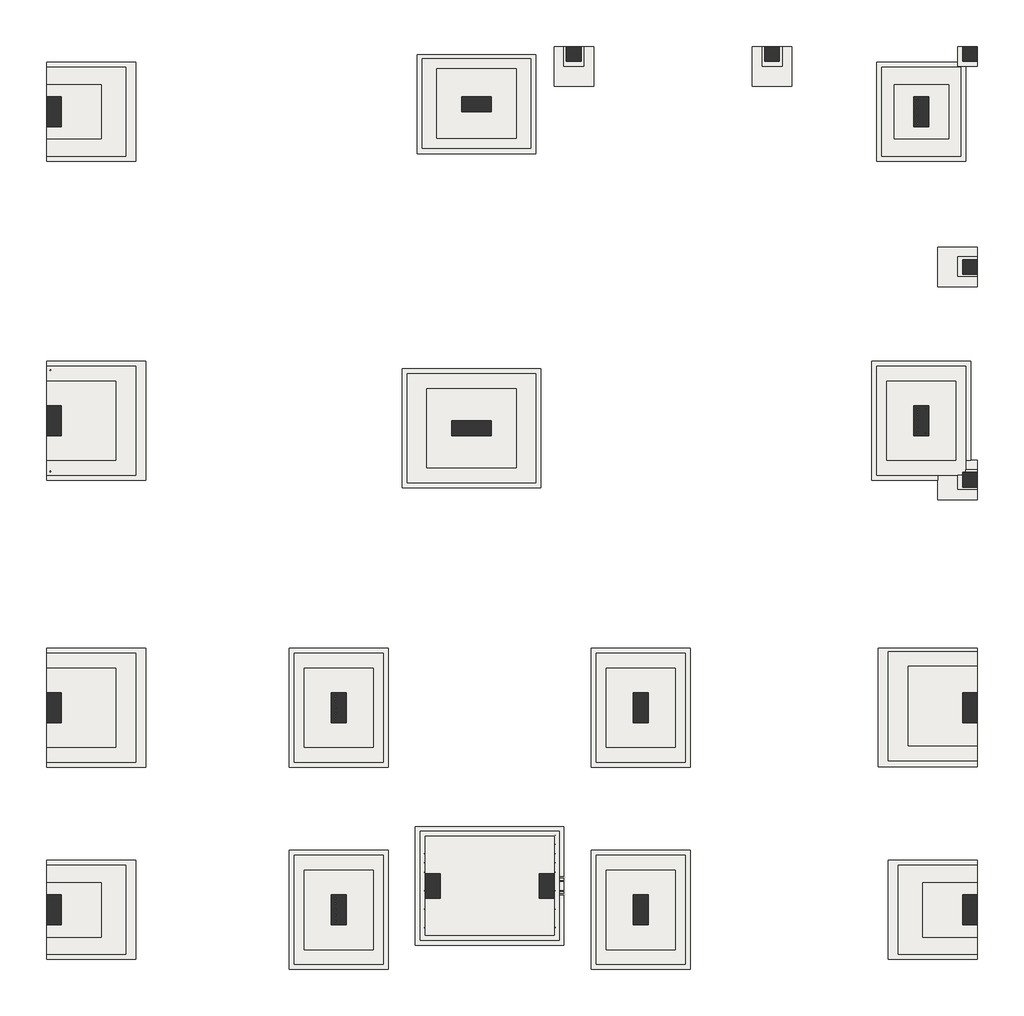
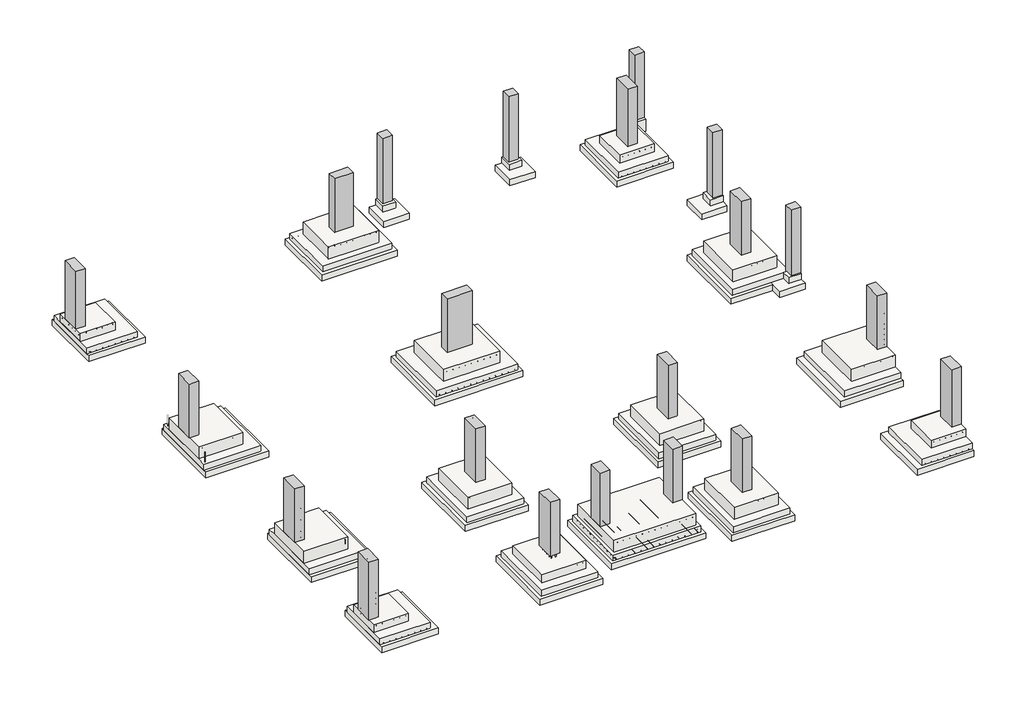
# One storey, part 1 of 6: 38 slabs, 21 columns.
"""IFC4 building model written with IfcOpenShell, lengths in millimetres."""

from ifc_helpers import new_model, si_unit, frame, origin, place, context, project, spatial, polyline, outline, extrude, faceted_brep, transform, mapped, element, save
from components import concrete_rectangular_column_c_1fc459bc

model = new_model("IFC4")

# Units and contexts
model_context = context("Model", 3, world=origin())
ifc_project = project(units=[si_unit("LENGTHUNIT", "METRE", prefix="MILLI")], contexts=[model_context])

# Site, building, storey
site = spatial("IfcSite", under=ifc_project)
building = spatial("IfcBuilding", under=site)
storey = spatial("IfcBuildingStorey", under=building, Elevation=-1828.8)

# Columns
placement = place(None, origin())
concrete_rectangular_column_c_shape = concrete_rectangular_column_c_1fc459bc(model_context)
element("IfcColumn", 1, ObjectType="Concrete-Rectangular-Column : C", at=placement, inside=storey, context=model_context, shape_type="MappedRepresentation", body=[
    mapped(concrete_rectangular_column_c_shape, transform((5670699.8650571, -3584604.6060698, 0.0), x_axis=(1.0, 0.0, 0.0), y_axis=(0.0, 1.0, 0.0), z_axis=(0.0, 0.0, 1.0))),
])
element("IfcColumn", 2, ObjectType="Concrete-Rectangular-Column : C", at=placement, inside=storey, context=model_context, shape_type="MappedRepresentation", body=[
    mapped(concrete_rectangular_column_c_shape, transform((5673747.8650571, -3584604.6060698, 0.0), x_axis=(1.0, 0.0, 0.0), y_axis=(0.0, 1.0, 0.0), z_axis=(0.0, 0.0, 1.0))),
])
element("IfcColumn", 3, ObjectType="Concrete-Rectangular-Column : C", at=placement, inside=storey, context=model_context, shape_type="MappedRepresentation", body=[
    mapped(concrete_rectangular_column_c_shape, transform((5676795.8650571, -3584604.6060698, 0.0), x_axis=(1.0, 0.0, 0.0), y_axis=(0.0, 1.0, 0.0), z_axis=(0.0, 0.0, 1.0))),
])
element("IfcColumn", 4, ObjectType="Concrete-Rectangular-Column : C", at=placement, inside=storey, context=model_context, shape_type="MappedRepresentation", body=[
    mapped(concrete_rectangular_column_c_shape, transform((5676795.8650571, -3587881.949152, 0.0), x_axis=(1.0, 0.0, 0.0), y_axis=(0.0, 1.0, 0.0), z_axis=(0.0, 0.0, 1.0))),
])
element("IfcColumn", 5, ObjectType="Concrete-Rectangular-Column : C", at=placement, inside=storey, context=model_context, shape_type="MappedRepresentation", body=[
    mapped(concrete_rectangular_column_c_shape, transform((5676795.8650571, -3591159.3007286, 0.0), x_axis=(1.0, 0.0, 0.0), y_axis=(0.0, 1.0, 0.0), z_axis=(0.0, 0.0, 1.0))),
])
element("IfcColumn", 6, ObjectType="Concrete-Rectangular-Column : C1", at=placement, inside=storey, context=model_context, shape_type="SweptSolid", body=[
    extrude(outline(polyline([(5662813.1113073, -3585265.1289932), (5662813.1113073, -3585722.3289932), (5662584.5113073, -3585722.3289932), (5662584.5113073, -3585265.1289932), (5662813.1113073, -3585265.1289932)])), frame((0.0, 0.0, -1473.2), z_axis=(0.0, 0.0, 1.0), x_axis=(1.0, 0.0, 0.0)), (0.0, 0.0, 1.0), 1473.2),
])
element("IfcColumn", 7, ObjectType="Concrete-Rectangular-Column : C1", at=placement, inside=storey, context=model_context, shape_type="SweptSolid", body=[
    extrude(outline(polyline([(5676160.8165246, -3585265.1224803), (5676160.8165246, -3585722.3224803), (5675932.2165246, -3585722.3224803), (5675932.2165246, -3585265.1224803), (5676160.8165246, -3585265.1224803)])), frame((0.0, 0.0, -1473.2), z_axis=(0.0, 0.0, 1.0), x_axis=(1.0, 0.0, 0.0)), (0.0, 0.0, 1.0), 1473.2),
])
element("IfcColumn", 8, ObjectType="Concrete-Rectangular-Column : C1", at=placement, inside=storey, context=model_context, shape_type="SweptSolid", body=[
    extrude(outline(polyline([(5662813.1113073, -3597545.8975754), (5662813.1113073, -3598003.0975754), (5662584.5113073, -3598003.0975754), (5662584.5113073, -3597545.8975754), (5662813.1113073, -3597545.8975754)])), frame((0.0, 0.0, -1473.2), z_axis=(0.0, 0.0, 1.0), x_axis=(1.0, 0.0, 0.0)), (0.0, 0.0, 1.0), 1473.2),
])
element("IfcColumn", 9, ObjectType="Concrete-Rectangular-Column : C1", at=placement, inside=storey, context=model_context, shape_type="SweptSolid", body=[
    extrude(outline(polyline([(5676910.1113073, -3597545.8975754), (5676910.1113073, -3598003.0975754), (5676681.5113073, -3598003.0975754), (5676681.5113073, -3597545.8975754), (5676910.1113073, -3597545.8975754)])), frame((0.0, 0.0, -1473.2), z_axis=(0.0, 0.0, 1.0), x_axis=(1.0, 0.0, 0.0)), (0.0, 0.0, 1.0), 1473.2),
])
element("IfcColumn", 10, ObjectType="Concrete-Rectangular-Column : C2", at=placement, inside=storey, context=model_context, shape_type="SweptSolid", body=[
    extrude(outline(polyline([(5668972.6206949, -3585265.1224803), (5669429.8206949, -3585265.1224803), (5669429.8206949, -3585493.7224803), (5668972.6206949, -3585493.7224803), (5668972.6206949, -3585265.1224803)])), frame((0.0, 0.0, -1371.6), z_axis=(0.0, 0.0, 1.0), x_axis=(1.0, 0.0, 0.0)), (0.0, 0.0, 1.0), 1371.6),
])
element("IfcColumn", 11, ObjectType="Concrete-Rectangular-Column : C2", at=placement, inside=storey, context=model_context, shape_type="SweptSolid", body=[
    extrude(outline(polyline([(5676160.8165246, -3590021.0682909), (5676160.8165246, -3590478.2682909), (5675932.2165246, -3590478.2682909), (5675932.2165246, -3590021.0682909), (5676160.8165246, -3590021.0682909)])), frame((0.0, 0.0, -1371.6), z_axis=(0.0, 0.0, 1.0), x_axis=(1.0, 0.0, 0.0)), (0.0, 0.0, 1.0), 1371.6),
])
element("IfcColumn", 12, ObjectType="Concrete-Rectangular-Column : C2", at=placement, inside=storey, context=model_context, shape_type="SweptSolid", body=[
    extrude(outline(polyline([(5662813.1650571, -3590021.0682909), (5662813.1650571, -3590478.2682909), (5662584.5650571, -3590478.2682909), (5662584.5650571, -3590021.0682909), (5662813.1650571, -3590021.0682909)])), frame((0.0, 0.0, -1371.6), z_axis=(0.0, 0.0, 1.0), x_axis=(1.0, 0.0, 0.0)), (0.0, 0.0, 1.0), 1371.6),
])
element("IfcColumn", 13, ObjectType="Concrete-Rectangular-Column : C2", at=placement, inside=storey, context=model_context, shape_type="SweptSolid", body=[
    extrude(outline(polyline([(5662813.1650571, -3594436.6523052), (5662813.1650571, -3594893.8523052), (5662584.5650571, -3594893.8523052), (5662584.5650571, -3594436.6523052), (5662813.1650571, -3594436.6523052)])), frame((0.0, 0.0, -1371.6), z_axis=(0.0, 0.0, 1.0), x_axis=(1.0, 0.0, 0.0)), (0.0, 0.0, 1.0), 1371.6),
])
element("IfcColumn", 14, ObjectType="Concrete-Rectangular-Column : C2", at=placement, inside=storey, context=model_context, shape_type="SweptSolid", body=[
    extrude(outline(polyline([(5667194.6165246, -3594436.6523052), (5667194.6165246, -3594893.8523052), (5666966.0165246, -3594893.8523052), (5666966.0165246, -3594436.6523052), (5667194.6165246, -3594436.6523052)])), frame((0.0, 0.0, -1371.6), z_axis=(0.0, 0.0, 1.0), x_axis=(1.0, 0.0, 0.0)), (0.0, 0.0, 1.0), 1371.6),
])
element("IfcColumn", 15, ObjectType="Concrete-Rectangular-Column : C2", at=placement, inside=storey, context=model_context, shape_type="SweptSolid", body=[
    extrude(outline(polyline([(5671842.8165246, -3594436.6523052), (5671842.8165246, -3594893.8523052), (5671614.2165246, -3594893.8523052), (5671614.2165246, -3594436.6523052), (5671842.8165246, -3594436.6523052)])), frame((0.0, 0.0, -1371.6), z_axis=(0.0, 0.0, 1.0), x_axis=(1.0, 0.0, 0.0)), (0.0, 0.0, 1.0), 1371.6),
])
element("IfcColumn", 16, ObjectType="Concrete-Rectangular-Column : C2", at=placement, inside=storey, context=model_context, shape_type="SweptSolid", body=[
    extrude(outline(polyline([(5676910.1650571, -3594436.6523052), (5676910.1650571, -3594893.8523052), (5676681.5650571, -3594893.8523052), (5676681.5650571, -3594436.6523052), (5676910.1650571, -3594436.6523052)])), frame((0.0, 0.0, -1371.6), z_axis=(0.0, 0.0, 1.0), x_axis=(1.0, 0.0, 0.0)), (0.0, 0.0, 1.0), 1371.6),
])
element("IfcColumn", 17, ObjectType="Concrete-Rectangular-Column : C2", at=placement, inside=storey, context=model_context, shape_type="SweptSolid", body=[
    extrude(outline(polyline([(5671842.8165246, -3597545.8975754), (5671842.8165246, -3598003.0975754), (5671614.2165246, -3598003.0975754), (5671614.2165246, -3597545.8975754), (5671842.8165246, -3597545.8975754)])), frame((0.0, 0.0, -1371.6), z_axis=(0.0, 0.0, 1.0), x_axis=(1.0, 0.0, 0.0)), (0.0, 0.0, 1.0), 1371.6),
])
element("IfcColumn", 18, ObjectType="Concrete-Rectangular-Column : C2", at=placement, inside=storey, context=model_context, shape_type="SweptSolid", body=[
    extrude(outline(polyline([(5667194.6165246, -3597545.8975754), (5667194.6165246, -3598003.0975754), (5666966.0165246, -3598003.0975754), (5666966.0165246, -3597545.8975754), (5667194.6165246, -3597545.8975754)])), frame((0.0, 0.0, -1371.6), z_axis=(0.0, 0.0, 1.0), x_axis=(1.0, 0.0, 0.0)), (0.0, 0.0, 1.0), 1371.6),
])
element("IfcColumn", 19, ObjectType="Concrete-Rectangular-Column : C3", at=placement, inside=storey, context=model_context, shape_type="SweptSolid", body=[
    extrude(outline(polyline([(5668820.2206949, -3590249.6682909), (5669429.8206949, -3590249.6682909), (5669429.8206949, -3590478.2682909), (5668820.2206949, -3590478.2682909), (5668820.2206949, -3590249.6682909)])), frame((0.0, 0.0, -1371.6), z_axis=(0.0, 0.0, 1.0), x_axis=(1.0, 0.0, 0.0)), (0.0, 0.0, 1.0), 1371.6),
])
element("IfcColumn", 20, ObjectType="Concrete-Rectangular-Column : C4", at=placement, inside=storey, context=model_context, shape_type="SweptSolid", body=[
    extrude(outline(polyline([(5668642.4165246, -3597217.2875145), (5668642.4165246, -3597598.2875145), (5668413.8165246, -3597598.2875145), (5668413.8165246, -3597217.2875145), (5668642.4165246, -3597217.2875145)])), frame((0.0, 0.0, -1371.6), z_axis=(0.0, 0.0, 1.0), x_axis=(1.0, 0.0, 0.0)), (0.0, 0.0, 1.0), 1371.6),
])
element("IfcColumn", 21, ObjectType="Concrete-Rectangular-Column : C4", at=placement, inside=storey, context=model_context, shape_type="SweptSolid", body=[
    extrude(outline(polyline([(5670395.0165245, -3597217.2875145), (5670395.0165245, -3597598.2875145), (5670166.4165245, -3597598.2875145), (5670166.4165245, -3597217.2875145), (5670395.0165245, -3597217.2875145)])), frame((0.0, 0.0, -1371.6), z_axis=(0.0, 0.0, 1.0), x_axis=(1.0, 0.0, 0.0)), (0.0, 0.0, 1.0), 1371.6),
])

# Slabs
element("IfcSlab", 22, ObjectType="Footing-Rectangular : F1", at=placement, inside=storey, context=model_context, shape_type="Brep", body=[
    faceted_brep([(5663803.7113073, -3584807.9113604, -1676.4), (5662584.5113073, -3584807.9113604, -1676.4), (5662584.5113073, -3585074.6113604, -1676.4), (5662584.5113073, -3585912.8113604, -1676.4), (5662584.5113073, -3586179.5113604, -1676.4), (5663803.7113073, -3586179.5113604, -1676.4), (5663803.7113073, -3584807.9113604, -1828.8), (5662584.5113073, -3584807.9113604, -1828.8), (5662584.5113073, -3586179.5113604, -1828.8), (5663803.7113073, -3586179.5113604, -1828.8)], [[[0, 1, 2, 3, 4, 5]], [[1, 0, 6, 7]], [[4, 3, 2, 1, 7, 8]], [[5, 4, 8, 9]], [[0, 5, 9, 6]], [[7, 6, 9, 8]]]),
])
element("IfcSlab", 23, ObjectType="Footing-Rectangular : F1", at=placement, inside=storey, context=model_context, shape_type="SweptSolid", body=[
    extrude(outline(polyline([(5675436.9165246, -3584807.9224803), (5676656.1165246, -3584807.9224803), (5676656.1165246, -3586179.5224803), (5675436.9165246, -3586179.5224803), (5675436.9165246, -3584807.9224803)])), frame((0.0, 0.0, -1828.8), z_axis=(0.0, 0.0, 1.0), x_axis=(1.0, 0.0, 0.0)), (0.0, 0.0, 1.0), 152.4),
])
element("IfcSlab", 24, ObjectType="Footing-Rectangular : F1", at=placement, inside=storey, context=model_context, shape_type="Brep", body=[
    faceted_brep([(5663803.7113073, -3597090.2875145, -1676.4), (5662584.5113073, -3597090.2875145, -1676.4), (5662584.5113073, -3597356.9875145, -1676.4), (5662584.5113073, -3598195.1875145, -1676.4), (5662584.5113073, -3598461.8875145, -1676.4), (5663803.7113073, -3598461.8875145, -1676.4), (5663803.7113073, -3597090.2875145, -1828.8), (5662584.5113073, -3597090.2875145, -1828.8), (5662584.5113073, -3598461.8875145, -1828.8), (5663803.7113073, -3598461.8875145, -1828.8)], [[[0, 1, 2, 3, 4, 5]], [[1, 0, 6, 7]], [[4, 3, 2, 1, 7, 8]], [[5, 4, 8, 9]], [[0, 5, 9, 6]], [[7, 6, 9, 8]]]),
])
element("IfcSlab", 25, ObjectType="Footing-Rectangular : F1", at=placement, inside=storey, context=model_context, shape_type="Brep", body=[
    faceted_brep([(5676910.1650571, -3597090.2875145, -1676.4), (5675690.9650571, -3597090.2875145, -1676.4), (5675690.9650571, -3598461.8875145, -1676.4), (5676910.1650571, -3598461.8875145, -1676.4), (5676910.1650571, -3598195.1875145, -1676.4), (5676910.1650571, -3597356.9875145, -1676.4), (5676910.1650571, -3597090.2875145, -1828.8), (5675690.9650571, -3597090.2875145, -1828.8), (5675690.9650571, -3598461.8875145, -1828.8), (5676910.1650571, -3598461.8875145, -1828.8)], [[[0, 1, 2, 3, 4, 5]], [[1, 0, 6, 7]], [[2, 1, 7, 8]], [[3, 2, 8, 9]], [[0, 5, 4, 3, 9, 6]], [[7, 6, 9, 8]]]),
])
element("IfcSlab", 26, ObjectType="Footing-Rectangular : F1 TOP", at=placement, inside=storey, context=model_context, shape_type="SweptSolid", body=[
    extrude(outline(polyline([(5662584.5113073, -3585074.6113604), (5663422.7113073, -3585074.6113604), (5663422.7113073, -3585912.8113604), (5662584.5113073, -3585912.8113604), (5662584.5113073, -3585074.6113604)])), frame((0.0, 0.0, -1676.4), z_axis=(0.0, 0.0, 1.0), x_axis=(1.0, 0.0, 0.0)), (0.0, 0.0, 1.0), 203.2),
])
element("IfcSlab", 27, ObjectType="Footing-Rectangular : F1 TOP", at=placement, inside=storey, context=model_context, shape_type="SweptSolid", body=[
    extrude(outline(polyline([(5675627.4165246, -3585912.8224803), (5675627.4165246, -3585074.6224803), (5676465.6165246, -3585074.6224803), (5676465.6165246, -3585912.8224803), (5675627.4165246, -3585912.8224803)])), frame((0.0, 0.0, -1676.4), z_axis=(0.0, 0.0, 1.0), x_axis=(1.0, 0.0, 0.0)), (0.0, 0.0, 1.0), 203.2),
])
element("IfcSlab", 28, ObjectType="Footing-Rectangular : F1 TOP", at=placement, inside=storey, context=model_context, shape_type="SweptSolid", body=[
    extrude(outline(polyline([(5662584.5113073, -3597356.9875145), (5663422.7113073, -3597356.9875145), (5663422.7113073, -3598195.1875145), (5662584.5113073, -3598195.1875145), (5662584.5113073, -3597356.9875145)])), frame((0.0, 0.0, -1676.4), z_axis=(0.0, 0.0, 1.0), x_axis=(1.0, 0.0, 0.0)), (0.0, 0.0, 1.0), 203.2),
])
element("IfcSlab", 29, ObjectType="Footing-Rectangular : F1 TOP", at=placement, inside=storey, context=model_context, shape_type="SweptSolid", body=[
    extrude(outline(polyline([(5676071.9650571, -3598195.1875145), (5676071.9650571, -3597356.9875145), (5676910.1650571, -3597356.9875145), (5676910.1650571, -3598195.1875145), (5676071.9650571, -3598195.1875145)])), frame((0.0, 0.0, -1676.4), z_axis=(0.0, 0.0, 1.0), x_axis=(1.0, 0.0, 0.0)), (0.0, 0.0, 1.0), 203.2),
])
element("IfcSlab", 30, ObjectType="Footing-Rectangular : F2", at=placement, inside=storey, context=model_context, shape_type="SweptSolid", body=[
    extrude(outline(polyline([(5668363.0297535, -3586052.5224803), (5668363.0297535, -3584680.9224803), (5670039.4297535, -3584680.9224803), (5670039.4297535, -3586052.5224803), (5668363.0297535, -3586052.5224803)])), frame((0.0, 0.0, -1828.8), z_axis=(0.0, 0.0, 1.0), x_axis=(1.0, 0.0, 0.0)), (0.0, 0.0, 1.0), 152.4),
])
element("IfcSlab", 31, ObjectType="Footing-Rectangular : F2", at=placement, inside=storey, context=model_context, shape_type="Brep", body=[
    faceted_brep([(5663956.1113073, -3589411.5284482, -1676.4), (5662584.5113073, -3589411.5284482, -1676.4), (5662584.5113073, -3589640.1284482, -1676.4), (5662584.5113073, -3590859.3284482, -1676.4), (5662584.5113073, -3591087.9284482, -1676.4), (5663956.1113073, -3591087.9284482, -1676.4), (5663956.1113073, -3589411.5284482, -1828.8), (5662584.5113073, -3589411.5284482, -1828.8), (5662584.5113073, -3591087.9284482, -1828.8), (5663956.1113073, -3591087.9284482, -1828.8)], [[[0, 1, 2, 3, 4, 5]], [[1, 0, 6, 7]], [[4, 3, 2, 1, 7, 8]], [[5, 4, 8, 9]], [[0, 5, 9, 6]], [[7, 6, 9, 8]]]),
])
element("IfcSlab", 32, ObjectType="Footing-Rectangular : F2", at=placement, inside=storey, context=model_context, shape_type="Brep", body=[
    faceted_brep([(5676732.3165246, -3589411.4682909, -1676.4), (5675360.7165246, -3589411.4682909, -1676.4), (5675360.7165246, -3591087.8682909, -1676.4), (5676605.3650571, -3591087.8682909, -1676.4), (5676732.3165246, -3591087.8682909, -1676.4), (5676732.3165246, -3591000.363802, -1676.4), (5676732.3165246, -3589411.4682909, -1828.8), (5675360.7165246, -3589411.4682909, -1828.8), (5675360.7165246, -3591087.8682909, -1828.8), (5676605.3650571, -3591087.8682909, -1828.8), (5676732.3165246, -3591087.8682909, -1828.8), (5676732.3165246, -3591000.363802, -1828.8)], [[[0, 1, 2, 3, 4, 5]], [[1, 0, 6, 7]], [[2, 1, 7, 8]], [[4, 3, 2, 8, 9, 10]], [[0, 5, 4, 10, 11, 6]], [[7, 6, 11, 10, 9, 8]]]),
])
element("IfcSlab", 33, ObjectType="Footing-Rectangular : F2", at=placement, inside=storey, context=model_context, shape_type="Brep", body=[
    faceted_brep([(5663956.1113073, -3593827.0523052, -1676.4), (5662584.5113073, -3593827.0523052, -1676.4), (5662584.5113073, -3594055.6523052, -1676.4), (5662584.5113073, -3595274.8523052, -1676.4), (5662584.5113073, -3595503.4523052, -1676.4), (5663956.1113073, -3595503.4523052, -1676.4), (5663956.1113073, -3593827.0523052, -1828.8), (5662584.5113073, -3593827.0523052, -1828.8), (5662584.5113073, -3595503.4523052, -1828.8), (5663956.1113073, -3595503.4523052, -1828.8)], [[[0, 1, 2, 3, 4, 5]], [[1, 0, 6, 7]], [[4, 3, 2, 1, 7, 8]], [[5, 4, 8, 9]], [[0, 5, 9, 6]], [[7, 6, 9, 8]]]),
])
element("IfcSlab", 34, ObjectType="Footing-Rectangular : F2", at=placement, inside=storey, context=model_context, shape_type="SweptSolid", body=[
    extrude(outline(polyline([(5666394.5165246, -3596937.8875145), (5667766.1165246, -3596937.8875145), (5667766.1165246, -3598614.2875145), (5666394.5165246, -3598614.2875145), (5666394.5165246, -3596937.8875145)])), frame((0.0, 0.0, -1828.8), z_axis=(0.0, 0.0, 1.0), x_axis=(1.0, 0.0, 0.0)), (0.0, 0.0, 1.0), 152.4),
])
element("IfcSlab", 35, ObjectType="Footing-Rectangular : F2", at=placement, inside=storey, context=model_context, shape_type="SweptSolid", body=[
    extrude(outline(polyline([(5671042.7165246, -3596937.8875145), (5672414.3165246, -3596937.8875145), (5672414.3165246, -3598614.2875145), (5671042.7165246, -3598614.2875145), (5671042.7165246, -3596937.8875145)])), frame((0.0, 0.0, -1828.8), z_axis=(0.0, 0.0, 1.0), x_axis=(1.0, 0.0, 0.0)), (0.0, 0.0, 1.0), 152.4),
])
element("IfcSlab", 36, ObjectType="Footing-Rectangular : F2", at=placement, inside=storey, context=model_context, shape_type="Brep", body=[
    faceted_brep([(5676910.1650571, -3593801.6523052, -1676.4), (5675538.5650571, -3593801.6523052, -1676.4), (5675538.5650571, -3595478.0523052, -1676.4), (5676910.1650571, -3595478.0523052, -1676.4), (5676910.1650571, -3595249.4523052, -1676.4), (5676910.1650571, -3594030.2523052, -1676.4), (5676910.1650571, -3593801.6523052, -1828.8), (5675538.5650571, -3593801.6523052, -1828.8), (5675538.5650571, -3595478.0523052, -1828.8), (5676910.1650571, -3595478.0523052, -1828.8)], [[[0, 1, 2, 3, 4, 5]], [[1, 0, 6, 7]], [[2, 1, 7, 8]], [[3, 2, 8, 9]], [[0, 5, 4, 3, 9, 6]], [[7, 6, 9, 8]]]),
])
element("IfcSlab", 37, ObjectType="Footing-Rectangular : F2", at=placement, inside=storey, context=model_context, shape_type="SweptSolid", body=[
    extrude(outline(polyline([(5666394.5165246, -3593827.0523052), (5667766.1165246, -3593827.0523052), (5667766.1165246, -3595503.4523052), (5666394.5165246, -3595503.4523052), (5666394.5165246, -3593827.0523052)])), frame((0.0, 0.0, -1828.8), z_axis=(0.0, 0.0, 1.0), x_axis=(1.0, 0.0, 0.0)), (0.0, 0.0, 1.0), 152.4),
])
element("IfcSlab", 38, ObjectType="Footing-Rectangular : F2", at=placement, inside=storey, context=model_context, shape_type="SweptSolid", body=[
    extrude(outline(polyline([(5671042.7165246, -3593827.0523052), (5672414.3165246, -3593827.0523052), (5672414.3165246, -3595503.4523052), (5671042.7165246, -3595503.4523052), (5671042.7165246, -3593827.0523052)])), frame((0.0, 0.0, -1828.8), z_axis=(0.0, 0.0, 1.0), x_axis=(1.0, 0.0, 0.0)), (0.0, 0.0, 1.0), 152.4),
])
element("IfcSlab", 39, ObjectType="Footing-Rectangular : F2 TOP", at=placement, inside=storey, context=model_context, shape_type="SweptSolid", body=[
    extrude(outline(polyline([(5668591.6297535, -3585900.1224803), (5668591.6297535, -3584833.3224803), (5669810.8297535, -3584833.3224803), (5669810.8297535, -3585900.1224803), (5668591.6297535, -3585900.1224803)])), frame((0.0, 0.0, -1676.4), z_axis=(0.0, 0.0, 1.0), x_axis=(1.0, 0.0, 0.0)), (0.0, 0.0, 1.0), 304.8),
])
element("IfcSlab", 40, ObjectType="Footing-Rectangular : F2 TOP", at=placement, inside=storey, context=model_context, shape_type="SweptSolid", body=[
    extrude(outline(polyline([(5663651.3113073, -3590859.3284482), (5662584.5113073, -3590859.3284482), (5662584.5113073, -3589640.1284482), (5663651.3113073, -3589640.1284482), (5663651.3113073, -3590859.3284482)])), frame((0.0, 0.0, -1676.4), z_axis=(0.0, 0.0, 1.0), x_axis=(1.0, 0.0, 0.0)), (0.0, 0.0, 1.0), 304.8),
])
element("IfcSlab", 41, ObjectType="Footing-Rectangular : F2 TOP", at=placement, inside=storey, context=model_context, shape_type="SweptSolid", body=[
    extrude(outline(polyline([(5675513.1165246, -3589640.0682909), (5676579.9165246, -3589640.0682909), (5676579.9165246, -3590859.2682909), (5675513.1165246, -3590859.2682909), (5675513.1165246, -3589640.0682909)])), frame((0.0, 0.0, -1676.4), z_axis=(0.0, 0.0, 1.0), x_axis=(1.0, 0.0, 0.0)), (0.0, 0.0, 1.0), 304.8),
])
element("IfcSlab", 42, ObjectType="Footing-Rectangular : F2 TOP", at=placement, inside=storey, context=model_context, shape_type="SweptSolid", body=[
    extrude(outline(polyline([(5662584.5113073, -3594055.6523052), (5663651.3113073, -3594055.6523052), (5663651.3113073, -3595274.8523052), (5662584.5113073, -3595274.8523052), (5662584.5113073, -3594055.6523052)])), frame((0.0, 0.0, -1676.4), z_axis=(0.0, 0.0, 1.0), x_axis=(1.0, 0.0, 0.0)), (0.0, 0.0, 1.0), 304.8),
])
element("IfcSlab", 43, ObjectType="Footing-Rectangular : F2 TOP", at=placement, inside=storey, context=model_context, shape_type="SweptSolid", body=[
    extrude(outline(polyline([(5666546.9165246, -3597166.4875145), (5667613.7165246, -3597166.4875145), (5667613.7165246, -3598385.6875145), (5666546.9165246, -3598385.6875145), (5666546.9165246, -3597166.4875145)])), frame((0.0, 0.0, -1676.4), z_axis=(0.0, 0.0, 1.0), x_axis=(1.0, 0.0, 0.0)), (0.0, 0.0, 1.0), 203.2),
])
element("IfcSlab", 44, ObjectType="Footing-Rectangular : F2 TOP", at=placement, inside=storey, context=model_context, shape_type="SweptSolid", body=[
    extrude(outline(polyline([(5671195.1165246, -3597166.4875145), (5672261.9165246, -3597166.4875145), (5672261.9165246, -3598385.6875145), (5671195.1165246, -3598385.6875145), (5671195.1165246, -3597166.4875145)])), frame((0.0, 0.0, -1676.4), z_axis=(0.0, 0.0, 1.0), x_axis=(1.0, 0.0, 0.0)), (0.0, 0.0, 1.0), 304.8),
])
element("IfcSlab", 45, ObjectType="Footing-Rectangular : F2 TOP", at=placement, inside=storey, context=model_context, shape_type="SweptSolid", body=[
    extrude(outline(polyline([(5675843.3650571, -3594030.2523052), (5676910.1650571, -3594030.2523052), (5676910.1650571, -3595249.4523052), (5675843.3650571, -3595249.4523052), (5675843.3650571, -3594030.2523052)])), frame((0.0, 0.0, -1676.4), z_axis=(0.0, 0.0, 1.0), x_axis=(1.0, 0.0, 0.0)), (0.0, 0.0, 1.0), 304.8),
])
element("IfcSlab", 46, ObjectType="Footing-Rectangular : F2 TOP", at=placement, inside=storey, context=model_context, shape_type="SweptSolid", body=[
    extrude(outline(polyline([(5666546.9165246, -3594055.6523052), (5667613.7165246, -3594055.6523052), (5667613.7165246, -3595274.8523052), (5666546.9165246, -3595274.8523052), (5666546.9165246, -3594055.6523052)])), frame((0.0, 0.0, -1676.4), z_axis=(0.0, 0.0, 1.0), x_axis=(1.0, 0.0, 0.0)), (0.0, 0.0, 1.0), 304.8),
])
element("IfcSlab", 47, ObjectType="Footing-Rectangular : F2 TOP", at=placement, inside=storey, context=model_context, shape_type="SweptSolid", body=[
    extrude(outline(polyline([(5671195.1165246, -3594055.6523052), (5672261.9165246, -3594055.6523052), (5672261.9165246, -3595274.8523052), (5671195.1165246, -3595274.8523052), (5671195.1165246, -3594055.6523052)])), frame((0.0, 0.0, -1676.4), z_axis=(0.0, 0.0, 1.0), x_axis=(1.0, 0.0, 0.0)), (0.0, 0.0, 1.0), 304.8),
])
element("IfcSlab", 48, ObjectType="Footing-Rectangular : F3", at=placement, inside=storey, context=model_context, shape_type="SweptSolid", body=[
    extrude(outline(polyline([(5668134.4297535, -3591202.2284482), (5668134.4297535, -3589525.8284482), (5670115.6297535, -3589525.8284482), (5670115.6297535, -3591202.2284482), (5668134.4297535, -3591202.2284482)])), frame((0.0, 0.0, -1828.8), z_axis=(0.0, 0.0, 1.0), x_axis=(1.0, 0.0, 0.0)), (0.0, 0.0, 1.0), 152.4),
])
element("IfcSlab", 49, ObjectType="Footing-Rectangular : F3 TOP", at=placement, inside=storey, context=model_context, shape_type="SweptSolid", body=[
    extrude(outline(polyline([(5668439.2297535, -3590973.6284482), (5668439.2297535, -3589754.4284482), (5669810.8297535, -3589754.4284482), (5669810.8297535, -3590973.6284482), (5668439.2297535, -3590973.6284482)])), frame((0.0, 0.0, -1676.4), z_axis=(0.0, 0.0, 1.0), x_axis=(1.0, 0.0, 0.0)), (0.0, 0.0, 1.0), 304.8),
])
element("IfcSlab", 50, ObjectType="Footing-Rectangular : F4", at=placement, inside=storey, context=model_context, shape_type="SweptSolid", body=[
    extrude(outline(polyline([(5668337.6165246, -3598245.9875145), (5668337.6165246, -3596569.5875145), (5670471.2165246, -3596569.5875145), (5670471.2165246, -3598245.9875145), (5668337.6165246, -3598245.9875145)])), frame((0.0, 0.0, -1828.8), z_axis=(0.0, 0.0, 1.0), x_axis=(1.0, 0.0, 0.0)), (0.0, 0.0, 1.0), 152.4),
])
element("IfcSlab", 51, ObjectType="Footing-Rectangular : F4 TOP", at=placement, inside=storey, context=model_context, shape_type="SweptSolid", body=[
    extrude(outline(polyline([(5668413.8165246, -3598169.7875145), (5668413.8165246, -3596645.7875145), (5670395.0165246, -3596645.7875145), (5670395.0165246, -3598169.7875145), (5668413.8165246, -3598169.7875145)])), frame((0.0, 0.0, -1676.4), z_axis=(0.0, 0.0, 1.0), x_axis=(1.0, 0.0, 0.0)), (0.0, 0.0, 1.0), 304.8),
])
element("IfcSlab", 52, ObjectType="Footing-Rectangular : FOOTING", at=placement, inside=storey, context=model_context, shape_type="SweptSolid", body=[
    extrude(outline(polyline([(5670547.4297535, -3584490.4224803), (5670852.2297535, -3584490.4224803), (5670852.2297535, -3584795.2224803), (5670547.4297535, -3584795.2224803), (5670547.4297535, -3584490.4224803)])), frame((0.0, 0.0, -1828.8), z_axis=(0.0, 0.0, 1.0), x_axis=(1.0, 0.0, 0.0)), (0.0, 0.0, 1.0), 152.4),
])
element("IfcSlab", 53, ObjectType="Footing-Rectangular : FOOTING", at=placement, inside=storey, context=model_context, shape_type="SweptSolid", body=[
    extrude(outline(polyline([(5673602.0019836, -3584490.4224803), (5673906.8019836, -3584490.4224803), (5673906.8019836, -3584795.2224803), (5673602.0019836, -3584795.2224803), (5673602.0019836, -3584490.4224803)])), frame((0.0, 0.0, -1828.8), z_axis=(0.0, 0.0, 1.0), x_axis=(1.0, 0.0, 0.0)), (0.0, 0.0, 1.0), 152.4),
])
element("IfcSlab", 54, ObjectType="Footing-Rectangular : FOOTING", at=placement, inside=storey, context=model_context, shape_type="SweptSolid", body=[
    extrude(outline(polyline([(5676605.3650571, -3587723.0122254), (5676910.1650571, -3587723.0122254), (5676910.1650571, -3588027.8122254), (5676605.3650571, -3588027.8122254), (5676605.3650571, -3587723.0122254)])), frame((0.0, 0.0, -1828.8), z_axis=(0.0, 0.0, 1.0), x_axis=(1.0, 0.0, 0.0)), (0.0, 0.0, 1.0), 152.4),
])
element("IfcSlab", 55, ObjectType="Footing-Rectangular : FOOTING", at=placement, inside=storey, context=model_context, shape_type="SweptSolid", body=[
    extrude(outline(polyline([(5676732.3165246, -3591000.363802), (5676910.1650571, -3591000.363802), (5676910.1650571, -3591305.163802), (5676605.3650571, -3591305.163802), (5676605.3650571, -3591087.8682909), (5676732.3165246, -3591087.8682909), (5676732.3165246, -3591000.363802)])), frame((0.0, 0.0, -1828.8), z_axis=(0.0, 0.0, 1.0), x_axis=(1.0, 0.0, 0.0)), (0.0, 0.0, 1.0), 152.4),
])
element("IfcSlab", 56, ObjectType="Footing-Rectangular : FOOTING", at=placement, inside=storey, context=model_context, shape_type="Brep", body=[
    faceted_brep([(5676910.1650571, -3584490.4224803, -1676.4), (5676605.3650571, -3584490.4224803, -1676.4), (5676605.3650571, -3584795.2224803, -1676.4), (5676910.1650571, -3584795.2224803, -1676.4), (5676910.1650571, -3584490.4224803, -1981.2), (5676910.1650571, -3584795.2224803, -1981.2), (5676732.3165246, -3584795.2224803, -1981.2), (5676732.3165246, -3584731.7289932, -1981.2), (5676605.3650571, -3584731.7289932, -1981.2), (5676605.3650571, -3584490.4224803, -1981.2), (5676605.3650571, -3584731.7289932, -1828.8), (5676605.3650571, -3584795.2224803, -1828.8), (5676732.3165246, -3584795.2224803, -1828.8), (5676732.3165246, -3584731.7289932, -1828.8)], [[[0, 1, 2, 3]], [[4, 5, 6, 7, 8, 9]], [[1, 0, 4, 9]], [[2, 1, 9, 8, 10, 11]], [[3, 2, 11, 12, 6, 5]], [[0, 3, 5, 4]], [[13, 12, 11, 10]], [[13, 7, 6, 12]], [[7, 13, 10, 8]]]),
])
element("IfcSlab", 57, ObjectType="PCC", at=placement, inside=storey, context=model_context, shape_type="Brep", body=[
    faceted_brep([(5663956.1113073, -3584731.7113604, -1981.2), (5663956.1113073, -3586255.7113604, -1981.2), (5662584.5113073, -3586255.7113604, -1981.2), (5662584.5113073, -3584731.7113604, -1981.2), (5663956.1113073, -3584731.7113604, -1828.8), (5662584.5113073, -3584731.7113604, -1828.8), (5662584.5113073, -3584807.9113604, -1828.8), (5662584.5113073, -3586179.5113604, -1828.8), (5662584.5113073, -3586255.7113604, -1828.8), (5663956.1113073, -3586255.7113604, -1828.8)], [[[0, 1, 2, 3]], [[4, 5, 6, 7, 8, 9]], [[1, 0, 4, 9]], [[2, 1, 9, 8]], [[3, 2, 8, 7, 6, 5]], [[0, 3, 5, 4]]]),
])
element("IfcSlab", 58, ObjectType="PCC", at=placement, inside=storey, context=model_context, shape_type="Brep", body=[
    faceted_brep([(5670115.6206949, -3584617.4224803, -1981.2), (5670115.6206949, -3586141.4224803, -1981.2), (5668286.8206949, -3586141.4224803, -1981.2), (5668286.8206949, -3584617.4224803, -1981.2), (5670115.6206949, -3584617.4224803, -1828.8), (5668286.8206949, -3584617.4224803, -1828.8), (5668286.8206949, -3586141.4224803, -1828.8), (5670115.6206949, -3586141.4224803, -1828.8)], [[[0, 1, 2, 3]], [[4, 5, 6, 7]], [[1, 0, 4, 7]], [[2, 1, 7, 6]], [[3, 2, 6, 5]], [[0, 3, 5, 4]]]),
    faceted_brep([(5675284.5165246, -3591164.0682909, -1981.2), (5675284.5165246, -3589335.2682909, -1981.2), (5676808.5165246, -3589335.2682909, -1981.2), (5676808.5165246, -3590854.4964814, -1981.2), (5676300.8086455, -3590854.4964814, -1981.2), (5676300.8086455, -3591164.0682909, -1981.2), (5676300.5650571, -3591164.0682909, -1981.2), (5675284.5165246, -3591164.0682909, -1828.8), (5676300.5650571, -3591164.0682909, -1828.8), (5676300.8086455, -3591164.0682909, -1828.8), (5676300.8086455, -3590854.4964814, -1828.8), (5676808.5165246, -3590854.4964814, -1828.8), (5676808.5165246, -3589335.2682909, -1828.8), (5675284.5165246, -3589335.2682909, -1828.8)], [[[0, 1, 2, 3, 4, 5, 6]], [[7, 8, 9, 10, 11, 12, 13]], [[1, 0, 7, 13]], [[2, 1, 13, 12]], [[3, 2, 12, 11]], [[0, 6, 5, 9, 8, 7]], [[4, 3, 11, 10]], [[5, 4, 10, 9]]]),
    faceted_brep([(5675386.1650571, -3595575.3283721, -1981.2), (5675386.1650571, -3593746.5283721, -1981.2), (5676910.1650571, -3593746.5283721, -1981.2), (5676910.1650571, -3595575.3283721, -1981.2), (5675386.1650571, -3595575.3283721, -1828.8), (5676910.1650571, -3595575.3283721, -1828.8), (5676910.1650571, -3595478.0523052, -1828.8), (5676910.1650571, -3593801.6523052, -1828.8), (5676910.1650571, -3593746.5283721, -1828.8), (5675386.1650571, -3593746.5283721, -1828.8)], [[[0, 1, 2, 3]], [[4, 5, 6, 7, 8, 9]], [[1, 0, 4, 9]], [[2, 1, 9, 8]], [[3, 2, 8, 7, 6, 5]], [[0, 3, 5, 4]]]),
    faceted_brep([(5676910.1650571, -3597008.3822736, -1981.2), (5676910.1650571, -3598532.3822736, -1981.2), (5675538.0601964, -3598532.3822736, -1981.2), (5675538.0601964, -3597008.3822736, -1981.2), (5676910.1650571, -3597008.3822736, -1828.8), (5675538.0601964, -3597008.3822736, -1828.8), (5675538.0601964, -3598532.3822736, -1828.8), (5676910.1650571, -3598532.3822736, -1828.8), (5676910.1650571, -3598461.8875145, -1828.8), (5676910.1650571, -3597090.2875145, -1828.8)], [[[0, 1, 2, 3]], [[4, 5, 6, 7, 8, 9]], [[1, 0, 4, 9, 8, 7]], [[2, 1, 7, 6]], [[3, 2, 6, 5]], [[0, 3, 5, 4]]]),
    faceted_brep([(5672490.5165246, -3596860.0975754, -1981.2), (5672490.5165246, -3598688.8975754, -1981.2), (5670966.5165246, -3598688.8975754, -1981.2), (5670966.5165246, -3596860.0975754, -1981.2), (5672490.5165246, -3596860.0975754, -1828.8), (5670966.5165246, -3596860.0975754, -1828.8), (5670966.5165246, -3598688.8975754, -1828.8), (5672490.5165246, -3598688.8975754, -1828.8)], [[[0, 1, 2, 3]], [[4, 5, 6, 7]], [[1, 0, 4, 7]], [[2, 1, 7, 6]], [[3, 2, 6, 5]], [[0, 3, 5, 4]]]),
    faceted_brep([(5672490.5165246, -3593750.8523052, -1981.2), (5672490.5165246, -3595579.6523052, -1981.2), (5670966.5165246, -3595579.6523052, -1981.2), (5670966.5165246, -3593750.8523052, -1981.2), (5672490.5165246, -3593750.8523052, -1828.8), (5670966.5165246, -3593750.8523052, -1828.8), (5670966.5165246, -3595579.6523052, -1828.8), (5672490.5165246, -3595579.6523052, -1828.8)], [[[0, 1, 2, 3]], [[4, 5, 6, 7]], [[1, 0, 4, 7]], [[2, 1, 7, 6]], [[3, 2, 6, 5]], [[0, 3, 5, 4]]]),
    faceted_brep([(5668261.4165246, -3598322.1875145, -1981.2), (5668261.4165246, -3596493.3875145, -1981.2), (5670547.4165246, -3596493.3875145, -1981.2), (5670547.4165246, -3598322.1875145, -1981.2), (5668261.4165246, -3598322.1875145, -1828.8), (5670547.4165246, -3598322.1875145, -1828.8), (5670547.4165246, -3596493.3875145, -1828.8), (5668261.4165246, -3596493.3875145, -1828.8)], [[[0, 1, 2, 3]], [[4, 5, 6, 7]], [[1, 0, 4, 7]], [[2, 1, 7, 6]], [[3, 2, 6, 5]], [[0, 3, 5, 4]]]),
    faceted_brep([(5667842.3165246, -3596860.0975754, -1981.2), (5667842.3165246, -3598688.8975754, -1981.2), (5666318.3165246, -3598688.8975754, -1981.2), (5666318.3165246, -3596860.0975754, -1981.2), (5667842.3165246, -3596860.0975754, -1828.8), (5666318.3165246, -3596860.0975754, -1828.8), (5666318.3165246, -3598688.8975754, -1828.8), (5667842.3165246, -3598688.8975754, -1828.8)], [[[0, 1, 2, 3]], [[4, 5, 6, 7]], [[1, 0, 4, 7]], [[2, 1, 7, 6]], [[3, 2, 6, 5]], [[0, 3, 5, 4]]]),
    faceted_brep([(5662584.5113073, -3598536.5187088, -1981.2), (5662584.5113073, -3597012.5187088, -1981.2), (5663956.1650571, -3597012.5187088, -1981.2), (5663956.1650571, -3598536.5187088, -1981.2), (5662584.5113073, -3598536.5187088, -1828.8), (5663956.1650571, -3598536.5187088, -1828.8), (5663956.1650571, -3597012.5187088, -1828.8), (5662584.5113073, -3597012.5187088, -1828.8), (5662584.5113073, -3597090.2875145, -1828.8), (5662584.5113073, -3598461.8875145, -1828.8)], [[[0, 1, 2, 3]], [[4, 5, 6, 7, 8, 9]], [[1, 0, 4, 9, 8, 7]], [[2, 1, 7, 6]], [[3, 2, 6, 5]], [[0, 3, 5, 4]]]),
    faceted_brep([(5662584.5113073, -3595579.7655499, -1981.2), (5662584.5113073, -3593750.9655499, -1981.2), (5664108.5650571, -3593750.9655499, -1981.2), (5664108.5650571, -3595579.7655499, -1981.2), (5662584.5113073, -3595579.7655499, -1828.8), (5664108.5650571, -3595579.7655499, -1828.8), (5664108.5650571, -3593750.9655499, -1828.8), (5662584.5113073, -3593750.9655499, -1828.8), (5662584.5113073, -3593827.0523052, -1828.8), (5662584.5113073, -3595503.4523052, -1828.8)], [[[0, 1, 2, 3]], [[4, 5, 6, 7, 8, 9]], [[1, 0, 4, 9, 8, 7]], [[2, 1, 7, 6]], [[3, 2, 6, 5]], [[0, 3, 5, 4]]]),
    faceted_brep([(5662584.5113073, -3591164.0682909, -1981.2), (5662584.5113073, -3589335.2682909, -1981.2), (5664108.5650571, -3589335.2682909, -1981.2), (5664108.5650571, -3591164.0682909, -1981.2), (5662584.5113073, -3591164.0682909, -1828.8), (5664108.5650571, -3591164.0682909, -1828.8), (5664108.5650571, -3589335.2682909, -1828.8), (5662584.5113073, -3589335.2682909, -1828.8), (5662584.5113073, -3589411.5284482, -1828.8), (5662584.5113073, -3591087.9284482, -1828.8)], [[[0, 1, 2, 3]], [[4, 5, 6, 7, 8, 9]], [[1, 0, 4, 9, 8, 7]], [[2, 1, 7, 6]], [[3, 2, 6, 5]], [[0, 3, 5, 4]]]),
    faceted_brep([(5670191.8207731, -3589449.6284482, -1981.2), (5670191.8207731, -3591278.4284482, -1981.2), (5668058.2207731, -3591278.4284482, -1981.2), (5668058.2207731, -3589449.6284482, -1981.2), (5670191.8207731, -3589449.6284482, -1828.8), (5668058.2207731, -3589449.6284482, -1828.8), (5668058.2207731, -3591278.4284482, -1828.8), (5670191.8207731, -3591278.4284482, -1828.8)], [[[0, 1, 2, 3]], [[4, 5, 6, 7]], [[1, 0, 4, 7]], [[2, 1, 7, 6]], [[3, 2, 6, 5]], [[0, 3, 5, 4]]]),
    faceted_brep([(5667842.3165246, -3593750.9416055, -1981.2), (5667842.3165246, -3595579.7416055, -1981.2), (5666318.3165246, -3595579.7416055, -1981.2), (5666318.3165246, -3593750.9416055, -1981.2), (5667842.3165246, -3593750.9416055, -1828.8), (5666318.3165246, -3593750.9416055, -1828.8), (5666318.3165246, -3595579.7416055, -1828.8), (5667842.3165246, -3595579.7416055, -1828.8)], [[[0, 1, 2, 3]], [[4, 5, 6, 7]], [[1, 0, 4, 7]], [[2, 1, 7, 6]], [[3, 2, 6, 5]], [[0, 3, 5, 4]]]),
    faceted_brep([(5670395.0297535, -3585099.9018226, -1981.2), (5670395.0297535, -3584490.4224803, -1981.2), (5671004.6650571, -3584490.4224803, -1981.2), (5671004.6650571, -3585099.9018226, -1981.2), (5670395.0297535, -3585099.9018226, -1828.8), (5671004.6650571, -3585099.9018226, -1828.8), (5671004.6650571, -3584490.4224803, -1828.8), (5670852.2297535, -3584490.4224803, -1828.8), (5670547.4297535, -3584490.4224803, -1828.8), (5670395.0297535, -3584490.4224803, -1828.8)], [[[0, 1, 2, 3]], [[4, 5, 6, 7, 8, 9]], [[1, 0, 4, 9]], [[2, 1, 9, 8, 7, 6]], [[3, 2, 6, 5]], [[0, 3, 5, 4]]]),
    faceted_brep([(5673443.0650571, -3585099.8975754, -1981.2), (5673443.0650571, -3584490.4224803, -1981.2), (5674052.6650571, -3584490.4224803, -1981.2), (5674052.6650571, -3585099.8975754, -1981.2), (5673443.0650571, -3585099.8975754, -1828.8), (5674052.6650571, -3585099.8975754, -1828.8), (5674052.6650571, -3584490.4224803, -1828.8), (5673906.8019836, -3584490.4224803, -1828.8), (5673602.0019836, -3584490.4224803, -1828.8), (5673443.0650571, -3584490.4224803, -1828.8)], [[[0, 1, 2, 3]], [[4, 5, 6, 7, 8, 9]], [[1, 0, 4, 9]], [[2, 1, 9, 8, 7, 6]], [[3, 2, 6, 5]], [[0, 3, 5, 4]]]),
    faceted_brep([(5676300.5650571, -3588186.7449048, -1981.2), (5676300.5650571, -3587577.1449048, -1981.2), (5676910.1650571, -3587577.1449048, -1981.2), (5676910.1650571, -3588186.7449048, -1981.2), (5676300.5650571, -3588186.7449048, -1828.8), (5676910.1650571, -3588186.7449048, -1828.8), (5676910.1650571, -3588027.8122254, -1828.8), (5676910.1650571, -3587723.0122254, -1828.8), (5676910.1650571, -3587577.1449048, -1828.8), (5676300.5650571, -3587577.1449048, -1828.8)], [[[0, 1, 2, 3]], [[4, 5, 6, 7, 8, 9]], [[1, 0, 4, 9]], [[2, 1, 9, 8]], [[3, 2, 8, 7, 6, 5]], [[0, 3, 5, 4]]]),
    faceted_brep([(5676732.3165246, -3584731.7289932, -1981.2), (5676732.3165246, -3584795.2224803, -1981.2), (5676732.3165246, -3586255.7289932, -1981.2), (5675360.7165246, -3586255.7289932, -1981.2), (5675360.7165246, -3584731.7289932, -1981.2), (5676605.3650571, -3584731.7289932, -1981.2), (5676732.3165246, -3584731.7289932, -1828.8), (5676605.3650571, -3584731.7289932, -1828.8), (5675360.7165246, -3584731.7289932, -1828.8), (5675360.7165246, -3586255.7289932, -1828.8), (5676732.3165246, -3586255.7289932, -1828.8), (5676732.3165246, -3584795.2224803, -1828.8)], [[[0, 1, 2, 3, 4, 5]], [[6, 7, 8, 9, 10, 11]], [[2, 1, 0, 6, 11, 10]], [[3, 2, 10, 9]], [[4, 3, 9, 8]], [[0, 5, 4, 8, 7, 6]]]),
])
element("IfcSlab", 59, ObjectType="PCC", at=placement, inside=storey, context=model_context, shape_type="Brep", body=[
    faceted_brep([(5676910.1650571, -3590854.4964814, -1981.2), (5676910.1650571, -3591464.0964814, -1981.2), (5676300.5650571, -3591464.0964814, -1981.2), (5676300.5650571, -3591164.0682909, -1981.2), (5676300.8086455, -3591164.0682909, -1981.2), (5676300.8086455, -3590854.4964814, -1981.2), (5676808.5165246, -3590854.4964814, -1981.2), (5676910.1650571, -3591464.0964814, -1828.8), (5676910.1650571, -3591305.163802, -1828.8), (5676910.1650571, -3591000.363802, -1828.8), (5676910.1650571, -3590854.4964814, -1828.8), (5676808.5165246, -3590854.4964814, -1828.8), (5676300.8086455, -3590854.4964814, -1828.8), (5676300.8086455, -3591164.0682909, -1828.8), (5676300.5650571, -3591164.0682909, -1828.8), (5676300.5650571, -3591464.0964814, -1828.8)], [[[0, 1, 2, 3, 4, 5, 6]], [[7, 8, 9, 10, 11, 12, 13, 14, 15]], [[2, 15, 14, 3]], [[10, 0, 6, 5, 12, 11]], [[1, 0, 10, 9, 8, 7]], [[2, 1, 7, 15]], [[13, 4, 3, 14]], [[4, 13, 12, 5]]]),
])

save(model, "model.ifc")

# Revit data of these elements
# Grids (mm)
#   "A": line (5678199.39, -3585265.122) -> (5661365.848, -3585265.122)
#   "B": line (5678164.243, -3590478.328) -> (5661365.663, -3590478.328)
#   "C": line (5678135.54, -3594436.652) -> (5661365.513, -3594436.652)
#   "E": line (5678110.406, -3598003.098) -> (5661365.381, -3598003.098)
#   "1": line (5662584.511, -3601203.94) -> (5662584.511, -3583283.929)
#   "2": line (5666966.017, -3601203.94) -> (5666966.017, -3583283.936)
#   "3": line (5668413.83, -3601203.94) -> (5668413.83, -3583283.936)
#   "4": line (5669429.821, -3602012.8) -> (5669429.821, -3583283.888)
#   "5": line (5670395.03, -3601203.94) -> (5670395.03, -3583283.888)
#   "6": line (5671842.817, -3601203.94) -> (5671842.817, -3583283.936)
#   "7": line (5676160.817, -3602012.8) -> (5676160.817, -3583283.936)
#   "8": line (5676910.165, -3601203.94) -> (5676910.165, -3583283.936)
#   "D": line (5678199.39, -3597598.288) -> (5661365.381, -3597598.288)
#   "F": line (5678199.39, -3584490.422) -> (5661365.848, -3584490.422)
# Type "Concrete-Rectangular-Column : C"
#   b = 228.6 mm
#   h = 228.6 mm
#   Structural Material [instance default] = Concrete, Cast-in-Place gray
# Type "Concrete-Rectangular-Column : C1"
#   b = 228.6 mm
#   h = 457.2 mm
#   Structural Material [instance default] = Concrete, Cast-in-Place gray
# Type "Concrete-Rectangular-Column : C2"
#   b = 228.6 mm
#   h = 457.2 mm
#   Structural Material [instance default] = Concrete, Cast-in-Place gray
# Type "Concrete-Rectangular-Column : C3"
#   b = 228.6 mm
#   h = 609.6 mm
#   Structural Material [instance default] = Concrete, Cast-in-Place gray
# Type "Concrete-Rectangular-Column : C4"
#   b = 228.6 mm
#   h = 381 mm
#   Structural Material [instance default] = Concrete, Cast-in-Place gray
# Type "Footing-Rectangular : F1"
#   Width = 1219.2 mm
#   Length = 1371.6 mm
#   Foundation Thickness = 203.2 mm
#   Structural Material [instance default] = Concrete - Cast-in-Place Concrete
#   Assembly Code = ""
# Type "Footing-Rectangular : F1 TOP"
#   Width = 838.2 mm
#   Length = 838.2 mm
#   Foundation Thickness = 254 mm
#   Structural Material [instance default] = Concrete - Cast-in-Place Concrete
#   Assembly Code = ""
# Type "Footing-Rectangular : F2"
#   Width = 1371.6 mm
#   Length = 1676.4 mm
#   Foundation Thickness = 304.8 mm
#   Structural Material [instance default] = Concrete - Cast-in-Place Concrete
#   Assembly Code = ""
# Type "Footing-Rectangular : F2 TOP"
#   Width = 1066.8 mm
#   Length = 1219.2 mm
#   Foundation Thickness = 457.2 mm
#   Structural Material [instance default] = Concrete - Cast-in-Place Concrete
#   Assembly Code = ""
# Type "Footing-Rectangular : F3"
#   Width = 1676.4 mm
#   Length = 1981.2 mm
#   Foundation Thickness = 304.8 mm
#   Structural Material [instance default] = Concrete - Cast-in-Place Concrete
#   Assembly Code = ""
# Type "Footing-Rectangular : F3 TOP"
#   Width = 1219.2 mm
#   Length = 1371.6 mm
#   Foundation Thickness = 609.6 mm
#   Structural Material [instance default] = Concrete - Cast-in-Place Concrete
#   Assembly Code = ""
# Type "Footing-Rectangular : F4"
#   Width = 1676.4 mm
#   Length = 2133.6 mm
#   Foundation Thickness = 304.8 mm
#   Structural Material [instance default] = Concrete - Cast-in-Place Concrete
#   Assembly Code = ""
# Type "Footing-Rectangular : F4 TOP"
#   Width = 1524 mm
#   Length = 1981.2 mm
#   Foundation Thickness = 609.6 mm
#   Structural Material [instance default] = Concrete - Cast-in-Place Concrete
#   Assembly Code = ""
# Type "Footing-Rectangular : FOOTING"
#   Width = 304.8 mm
#   Length = 304.8 mm
#   Foundation Thickness = 304.8 mm
#   Structural Material [instance default] = Concrete - Cast-in-Place Concrete
#   Assembly Code = ""
# Type "PCC"
#   Layers, outside or top first: 152.4 mm "Concrete" (function 1)
# Elements 1, 2, 3, 4, 5 (IfcColumn, "Concrete-Rectangular-Column : C")
#   Structural Material = Concrete, Cast-in-Place gray
#   Phase Created = New Construction
#   Materials on its faces: "Concrete, Cast-in-Place gray"
# Elements 6, 7, 8, 9 (IfcColumn, "Concrete-Rectangular-Column : C1")
#   Structural Material = Concrete, Cast-in-Place gray
#   Phase Created = New Construction
#   Materials on its faces: "Concrete, Cast-in-Place gray"
# Elements 10, 11, 12, 13, 14, 15, 16, 17, 18 (IfcColumn, "Concrete-Rectangular-Column : C2")
#   Structural Material = Concrete, Cast-in-Place gray
#   Phase Created = New Construction
#   Materials on its faces: "Concrete, Cast-in-Place gray"
# Element 19 (IfcColumn, "Concrete-Rectangular-Column : C3")
#   Structural Material = Concrete, Cast-in-Place gray
#   Phase Created = New Construction
#   Materials on its faces: "Concrete, Cast-in-Place gray"
# Elements 20, 21 (IfcColumn, "Concrete-Rectangular-Column : C4")
#   Structural Material = Concrete, Cast-in-Place gray
#   Phase Created = New Construction
#   Materials on its faces: "Concrete, Cast-in-Place gray"
# Elements 22, 23, 24, 25 (IfcSlab, "Footing-Rectangular : F1")
#   Structural Material = Concrete - Cast-in-Place Concrete
#   Phase Created = New Construction
#   Materials on its faces: "Concrete - Cast-in-Place Concrete"
# Elements 26, 27, 28, 29 (IfcSlab, "Footing-Rectangular : F1 TOP")
#   Structural Material = Concrete - Cast-in-Place Concrete
#   Phase Created = New Construction
#   Materials on its faces: "Concrete - Cast-in-Place Concrete"
# Elements 30, 31, 32, 33, 34, 35, 36, 37, 38 (IfcSlab, "Footing-Rectangular : F2")
#   Structural Material = Concrete - Cast-in-Place Concrete
#   Phase Created = New Construction
#   Materials on its faces: "Concrete - Cast-in-Place Concrete"
# Elements 39, 40, 41, 42, 43, 44, 45, 46, 47 (IfcSlab, "Footing-Rectangular : F2 TOP")
#   Structural Material = Concrete - Cast-in-Place Concrete
#   Phase Created = New Construction
#   Materials on its faces: "Concrete - Cast-in-Place Concrete"
# Element 48 (IfcSlab, "Footing-Rectangular : F3")
#   Structural Material = Concrete - Cast-in-Place Concrete
#   Phase Created = New Construction
#   Materials on its faces: "Concrete - Cast-in-Place Concrete"
# Element 49 (IfcSlab, "Footing-Rectangular : F3 TOP")
#   Structural Material = Concrete - Cast-in-Place Concrete
#   Phase Created = New Construction
#   Materials on its faces: "Concrete - Cast-in-Place Concrete"
# Element 50 (IfcSlab, "Footing-Rectangular : F4")
#   Structural Material = Concrete - Cast-in-Place Concrete
#   Phase Created = New Construction
#   Materials on its faces: "Concrete - Cast-in-Place Concrete"
# Element 51 (IfcSlab, "Footing-Rectangular : F4 TOP")
#   Structural Material = Concrete - Cast-in-Place Concrete
#   Phase Created = New Construction
#   Materials on its faces: "Concrete - Cast-in-Place Concrete"
# Elements 52, 53, 54, 55, 56 (IfcSlab, "Footing-Rectangular : FOOTING")
#   Structural Material = Concrete - Cast-in-Place Concrete
#   Phase Created = New Construction
#   Materials on its faces: "Concrete - Cast-in-Place Concrete"
# Elements 57, 58 (IfcSlab, "PCC")
#   Height Offset From Level = 0 mm
#   Phase Created = New Construction
#   Materials on its faces: "Concrete"
# Element 59 (IfcSlab, "PCC")
#   built-in parameter 1001955 = 3.14159 (stored number, unit not read)
#   Height Offset From Level = 0 mm
#   Phase Created = New Construction
#   Materials on its faces: "Concrete"
# Materials
#   "Concrete, Cast-in-Place gray": class "Concrete", colour RGB 192 192 192, transparency 0, Description = "Cast-in-place concrete", Cost = 0
#   "Concrete - Cast-in-Place Concrete": class "Concrete", colour RGB 192 192 192, transparency 0, Cost = 0
#   "Concrete": class "Concrete", colour RGB 0 0 0, transparency 0, Description = "Portland Cement Concrete", Cost = 0
